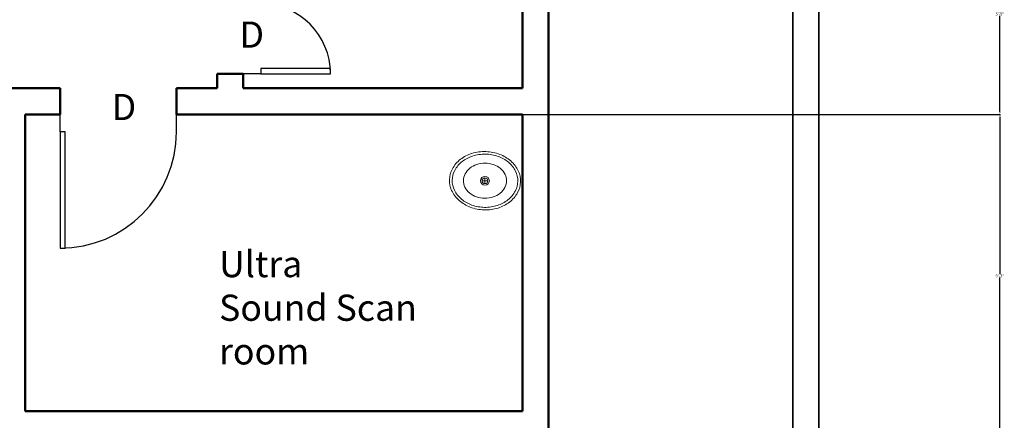
# Model space of a CAD drawing. Units: inches. Extents: x -364 to 705, y -52 to 1250.
# Tile 30 of 34: x 366 to 704, y 648 to 786. Entities that reach past the tile are written whole.
import ezdxf

# ---------------------------------------------------------------- set-up
doc = ezdxf.new("R2010")
doc.units = ezdxf.units.IN
doc.header["$MEASUREMENT"] = 0
for name, color, linetype, lineweight in [('A-ANNO-DIMS', 4, 'Continuous', 18), ('A-ANNO-IDEN', 1, 'Continuous', 18), ('A-AREA-IDEN', 3, 'Continuous', 18), ('A-DOOR', 1, 'Continuous', 25), ('A-FLOR-FIXT', 9, 'Continuous', 18), ('A-WALL', 41, 'Continuous', 50), ('C-WALL', 41, 'Continuous', 35)]:
    doc.layers.add(name, color=color, linetype=linetype, lineweight=lineweight)
doc.styles.get("Standard").update_dxf_attribs({"font": 'arial.ttf'})
doc.dimstyles.get("Standard").update_dxf_attribs({"dimtxt": 1, "dimasz": 1, "dimexe": 0.18, "dimexo": 0.0625, "dimgap": 0.09, "dimtad": 0, "dimtih": 1, "dimtoh": 1, "dimdec": 0, "dimzin": 0, "dimdsep": 46, "dimlunit": 3, "dimtxsty": 'Standard', "dimcen": 0.09, "dimadec": 0, "dimazin": 0, "dimtfac": 1, "dimtdec": 0, "dimtofl": 0, "dimtmove": 0, "dimatfit": 3, "dimfxl": 1, "dimtolj": 1, "dimtzin": 0, "dimarcsym": 0})

# ---------------------------------------------------------------- blocks, each defined once
blk = doc.blocks.new('*U3')
for p, q in [((0, 0), (0, -6)), ((-24, 0), (-24, -6))]:
    blk.add_line(p, q)
blk.add_lwpolyline([(0, 0), (0, 24), (-1.75, 24), (-1.75, 0)], close=True)
blk.add_arc((0, 0), 24, 90, 180)
blk = doc.blocks.new('*U4')
for p, q in [((0, 0), (0, 6)), ((40, 0), (40, 6))]:
    blk.add_line(p, q)
blk.add_lwpolyline([(0, 0), (0, -40), (1.75, -40), (1.75, 0)], close=True)
blk.add_arc((0, 0), 40, 270, 0)
blk = doc.blocks.new('Sink - Oval top')
for p, q in [((-1, 0), (1, 0)), ((0, 1), (0, -1))]:
    blk.add_line(p, q)
for points in [[(-12.23, 0.39, 0.117634), (-11.46, -3.36, 0.104469), (-8.88, -6.8, 0.090016), (-5.08, -9.07, 0.08192), (-0.32, -10.02, 0.08192), (4.49, -9.38, 0.090016), (8.42, -7.36, 0.104469), (11.22, -4.09, 0.117634), (12.23, -0.39, 0.117634), (11.46, 3.36, 0.104469), (8.88, 6.8, 0.090016), (5.08, 9.07, 0.08192), (0.32, 10.02, 0.08192), (-4.49, 9.38, 0.090016), (-8.42, 7.36, 0.104469), (-11.22, 4.09, 0.117634)], [(-11.29, 0.16, 0.118622), (-10.52, -3.25, 0.104678), (-8.07, -6.36, 0.089562), (-4.54, -8.37, 0.081185), (-0.13, -9.15, 0.081185), (4.3, -8.49, 0.089562), (7.89, -6.58, 0.104678), (10.42, -3.55, 0.118622), (11.29, -0.16, 0.118622), (10.52, 3.25, 0.104678), (8.07, 6.36, 0.089562), (4.54, 8.37, 0.081185), (0.13, 9.15, 0.081185), (-4.3, 8.49, 0.089562), (-7.89, 6.58, 0.104678), (-10.42, 3.55, 0.118622)], [(-7.42, 0.08, 0.118283), (-6.91, -2.17, 0.104607), (-5.29, -4.21, 0.089718), (-2.97, -5.53, 0.081436), (-0.07, -6.04, 0.081436), (2.84, -5.59, 0.089718), (5.2, -4.33, 0.104607), (6.86, -2.32, 0.118283), (7.42, -0.08, 0.118283), (6.91, 2.17, 0.104607), (5.29, 4.21, 0.089718), (2.97, 5.53, 0.081436), (0.07, 6.04, 0.081436), (-2.84, 5.59, 0.089718), (-5.2, 4.33, 0.104607), (-6.86, 2.32, 0.118283)]]:
    blk.add_lwpolyline(points, format="xyb", close=True)
for radius in [1.5, 1]:
    blk.add_circle((0, 0), radius)
blk = doc.blocks.new('*D82')
at = {"layer": 'A-ANNO-DIMS', "color": 0, "lineweight": -2, "transparency": 16777216}
for p, q in [((538.64, 753.11), (703.01, 753.11)), ((702.83, 752.11), (702.83, 698.22)), ((702.83, 643.11), (702.83, 697.01)), ((538.64, 642.11), (703.01, 642.11))]:
    blk.add_line(p, q, dxfattribs=at)
at = {"layer": 'A-ANNO-DIMS', "color": 0, "transparency": 16777216}
for points in [[(702.66, 752.11), (703, 752.11), (702.83, 753.11)], [(702.66, 643.11), (703, 643.11), (702.83, 642.11)]]:
    blk.add_solid(points, dxfattribs=at)
at = {"layer": 'Defpoints', "color": 0, "transparency": 16777216}
for p in [(538.58, 753.11), (702.83, 753.11), (538.58, 642.11)]:
    blk.add_point(p, dxfattribs=at)
at = {"layer": 'A-ANNO-DIMS', "color": 0, "transparency": 16777216, "insert": (702.83, 697.61), "char_height": 1, "attachment_point": 5}
blk.add_mtext('\\A1;9\'-3"', dxfattribs=at)
blk = doc.blocks.new('*D83')
at = {"layer": 'A-ANNO-DIMS', "color": 0, "lineweight": -2, "transparency": 16777216}
for p, q in [((538.64, 822.11), (703.01, 822.11)), ((702.83, 821.11), (702.83, 788.22)), ((702.83, 754.11), (702.83, 787.01)), ((538.64, 753.11), (703.01, 753.11))]:
    blk.add_line(p, q, dxfattribs=at)
at = {"layer": 'A-ANNO-DIMS', "color": 0, "transparency": 16777216}
for points in [[(702.66, 821.11), (703, 821.11), (702.83, 822.11)], [(702.66, 754.11), (703, 754.11), (702.83, 753.11)]]:
    blk.add_solid(points, dxfattribs=at)
at = {"layer": 'Defpoints', "color": 0, "transparency": 16777216}
for p in [(538.58, 822.11), (702.83, 822.11), (538.58, 753.11)]:
    blk.add_point(p, dxfattribs=at)
at = {"layer": 'A-ANNO-DIMS', "color": 0, "transparency": 16777216, "insert": (702.83, 787.61), "char_height": 1, "attachment_point": 5}
blk.add_mtext('\\A1;5\'-9"', dxfattribs=at)

msp = doc.modelspace()

# ---------------------------------------------------------------- linework, layer by layer
at = {"layer": 'A-WALL'}
for p, q in [((547.58, 11.11), (547.58, 986.11)), ((538.58, 762.11), (538.58, 822.11)), ((433.58, 762.11), (433.58, 767.11)), ((442.58, 767.11), (433.58, 767.11)), ((442.58, 762.11), (442.58, 767.11)), ((379.58, 762.11), (184.58, 762.11)), ((379.58, 762.11), (379.58, 753.11)), ((433.58, 762.11), (419.58, 762.11)), ((419.58, 753.11), (419.58, 762.11)), ((538.58, 762.11), (442.58, 762.11)), ((367.58, 651.11), (367.58, 753.11)), ((379.58, 753.11), (367.58, 753.11)), ((538.58, 753.11), (419.58, 753.11)), ((538.58, 651.11), (538.58, 753.11)), ((538.58, 651.11), (367.58, 651.11)), ((379.58, 651.11), (367.58, 651.11))]:
    msp.add_line(p, q, dxfattribs=at)
at = {"layer": 'C-WALL'}
for p, q in [((640.58, 11.11), (640.58, 1079.11)), ((631.58, 11.11), (631.58, 1070.11))]:
    msp.add_line(p, q, dxfattribs=at)

# ---------------------------------------------------------------- block references
at = {"layer": 'A-DOOR', "rotation": 270}
msp.add_blockref('*U3', (448.58, 767.11), dxfattribs=at)
at = {"layer": 'A-DOOR'}
msp.add_blockref('*U4', (379.58, 747.11), dxfattribs=at)
at = {"layer": 'A-FLOR-FIXT'}
msp.add_blockref('Sink - Oval top', (525.72, 730.3), dxfattribs=at)

# ---------------------------------------------------------------- texts
at = {"layer": 'A-ANNO-IDEN', "char_height": 9, "attachment_point": 1}
for insert in [(441.3, 785.04), (397.31, 760.13)]:
    msp.add_mtext_dynamic_manual_height_columns('D', width=17.6397, gutter_width=1, heights=[0], dxfattribs=dict(at, insert=insert))
at = {"layer": 'A-AREA-IDEN', "insert": (434.26, 706.14), "char_height": 9, "attachment_point": 1}
msp.add_mtext_dynamic_manual_height_columns('Ultra Sound Scan room', width=68.24, gutter_width=1, heights=[0], dxfattribs=at)

# ---------------------------------------------------------------- dimensions: what is measured, and where the dimension line sits
at = {"layer": 'A-ANNO-DIMS'}
for base, p1, p2, picture, middle in [((702.83, 822.11), (538.58, 753.11), (538.58, 822.11), '*D83', (702.83, 787.61)), ((702.83, 753.11), (538.58, 642.11), (538.58, 753.11), '*D82', (702.83, 697.61))]:
    dim = msp.add_linear_dim(base=base, p1=p1, p2=p2, angle=90, dimstyle='Standard', override={"dimdec": 1, "dimlfac": 1, "dimrnd": 0, "dimzin": 1, "dimdsep": 46, "dimlunit": 4, "dimfrac": 2}, dxfattribs=at)
    dim.commit()
    dim.dimension.update_dxf_attribs({"geometry": picture, "text_midpoint": middle})

doc.saveas('drawing.dxf')
